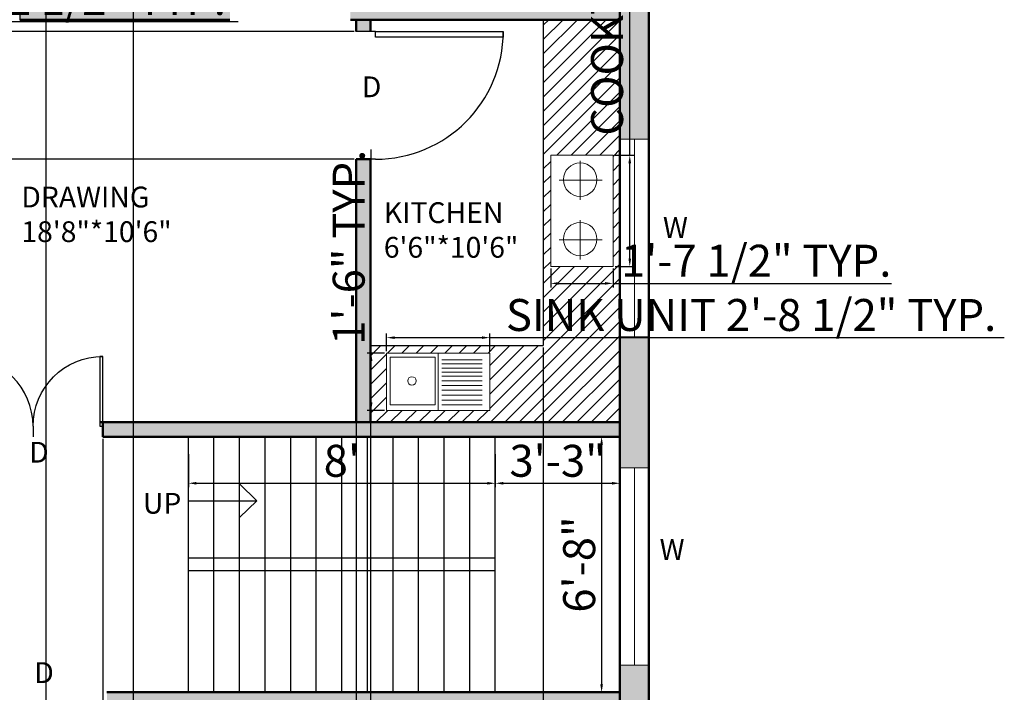
# Model space of a CAD drawing. Units: inches. Extents: x 1935 to 2445, y 1978 to 2806.
# Tile 3 of 4: x 2137 to 2445, y 2344 to 2554. Entities that reach past the tile are written whole.
import ezdxf

# ---------------------------------------------------------------- set-up
doc = ezdxf.new("R2010")
doc.units = ezdxf.units.IN
for name, color, linetype, lineweight in [('A-ANNO-DIMS', 2, 'Continuous', 18), ('A-ANNO-TEXT', 7, 'Continuous', 25), ('A-AREA-IDEN', 130, 'Continuous', 25), ('A-DOOR', 3, 'Continuous', 25), ('A-EQPM', 8, 'Continuous', 18), ('A-FLOR-CASE', 123, 'Continuous', 25), ('A-FLOR-CASE-PATT', 123, 'Continuous', 13), ('A-FLOR-FIXT', 9, 'Continuous', 18), ('A-FLOR-STRS', 7, 'Continuous', 25), ('A-GLAZ', 4, 'Continuous', 18), ('A-WALL-PATT', 225, 'Continuous', 13), ('WALL', 225, 'Continuous', 50)]:
    doc.layers.add(name, color=color, linetype=linetype, lineweight=lineweight)
doc.styles.get("Standard").update_dxf_attribs({"font": 'arial.ttf'})
doc.dimstyles.new('ISO-25', dxfattribs={"dimtxt": 10, "dimasz": 2.5, "dimexe": 1.25, "dimexo": 0.625, "dimtad": 1, "dimdec": 0, "dimlunit": 4, "dimtxsty": 'Standard', "dimcen": 2.5, "dimadec": 0, "dimazin": 0, "dimtfac": 1, "dimtdec": 0, "dimtmove": 0, "dimatfit": 3, "dimfxl": 1, "dimarcsym": 0})

# ---------------------------------------------------------------- blocks, each defined once
blk = doc.blocks.new('*U2')
for p, q in [((0, 0), (0, -6)), ((40, 0), (40, -6))]:
    blk.add_line(p, q)
blk.add_lwpolyline([(0, 0), (0, 40), (1.75, 40), (1.75, 0)], close=True)
blk.add_arc((0, 0), 40, 0, 90)
blk = doc.blocks.new('*D5')
at = {"layer": 'A-ANNO-DIMS', "color": 0, "lineweight": -2, "transparency": 16777216}
for p, q in [((2190.18, 2418.42), (2190.18, 2408.06)), ((2286.18, 2418.42), (2286.18, 2408.06)), ((2192.68, 2409.31), (2283.68, 2409.31))]:
    blk.add_line(p, q, dxfattribs=at)
at = {"layer": 'A-ANNO-DIMS', "color": 0, "lineweight": 100, "transparency": 16777216}
for points in [[(2192.68, 2409.72), (2192.68, 2408.89), (2190.18, 2409.31)], [(2283.68, 2409.72), (2283.68, 2408.89), (2286.18, 2409.31)]]:
    blk.add_solid(points, dxfattribs=at)
at = {"layer": 'Defpoints', "color": 0, "lineweight": 100, "transparency": 16777216}
for p in [(2190.18, 2419.04), (2286.18, 2419.04), (2286.18, 2409.31)]:
    blk.add_point(p, dxfattribs=at)
at = {"layer": 'A-ANNO-DIMS', "color": 0, "transparency": 16777216, "insert": (2238.18, 2415.04), "char_height": 10, "attachment_point": 5}
blk.add_mtext("8'", dxfattribs=at)
blk = doc.blocks.new('*D6')
at = {"layer": 'A-ANNO-DIMS', "color": 0, "lineweight": -2, "transparency": 16777216}
for p, q in [((2286.18, 2418.22), (2286.18, 2408.06)), ((2325.18, 2418.22), (2325.18, 2408.06)), ((2288.68, 2409.31), (2322.68, 2409.31))]:
    blk.add_line(p, q, dxfattribs=at)
at = {"layer": 'A-ANNO-DIMS', "color": 0, "lineweight": 100, "transparency": 16777216}
for points in [[(2288.68, 2409.72), (2288.68, 2408.89), (2286.18, 2409.31)], [(2322.68, 2409.72), (2322.68, 2408.89), (2325.18, 2409.31)]]:
    blk.add_solid(points, dxfattribs=at)
at = {"layer": 'Defpoints', "color": 0, "lineweight": 100, "transparency": 16777216}
for p in [(2286.18, 2418.85), (2325.18, 2418.85), (2325.18, 2409.31)]:
    blk.add_point(p, dxfattribs=at)
at = {"layer": 'A-ANNO-DIMS', "color": 0, "transparency": 16777216, "insert": (2305.68, 2415.04), "char_height": 10, "attachment_point": 5}
blk.add_mtext('3\'-3"', dxfattribs=at)
blk = doc.blocks.new('*D7')
at = {"layer": 'A-ANNO-DIMS', "color": 0, "lineweight": -2, "transparency": 16777216}
for p, q in [((2324.56, 2423.88), (2318.18, 2423.88)), ((2319.43, 2421.38), (2319.43, 2346.38)), ((2324.56, 2343.88), (2318.18, 2343.88))]:
    blk.add_line(p, q, dxfattribs=at)
at = {"layer": 'A-ANNO-DIMS', "color": 0, "lineweight": 100, "transparency": 16777216}
for points in [[(2319.01, 2421.38), (2319.85, 2421.38), (2319.43, 2423.88)], [(2319.01, 2346.38), (2319.85, 2346.38), (2319.43, 2343.88)]]:
    blk.add_solid(points, dxfattribs=at)
at = {"layer": 'Defpoints', "color": 0, "lineweight": 100, "transparency": 16777216}
for p in [(2325.18, 2423.88), (2319.43, 2343.88), (2325.18, 2343.88)]:
    blk.add_point(p, dxfattribs=at)
at = {"layer": 'A-ANNO-DIMS', "color": 0, "transparency": 16777216, "insert": (2313.7, 2383.88), "char_height": 10, "attachment_point": 5, "rotation": 90}
blk.add_mtext('6\'-8"', dxfattribs=at)
blk = doc.blocks.new('*D9')
at = {"layer": 'A-ANNO-DIMS', "color": 0, "lineweight": -2, "transparency": 16777216}
for p, q in [((2333.56, 2697.88), (1952.98, 2697.88)), ((1954.23, 2076.38), (1954.23, 2695.38)), ((2333.56, 2073.88), (1952.98, 2073.88))]:
    blk.add_line(p, q, dxfattribs=at)
at = {"layer": 'A-ANNO-DIMS', "color": 0, "lineweight": 100, "transparency": 16777216}
for points in [[(1953.82, 2695.38), (1954.65, 2695.38), (1954.23, 2697.88)], [(1953.82, 2076.38), (1954.65, 2076.38), (1954.23, 2073.88)]]:
    blk.add_solid(points, dxfattribs=at)
at = {"layer": 'Defpoints', "color": 0, "lineweight": 100, "transparency": 16777216}
for p in [(1954.23, 2697.88), (2334.18, 2697.88), (2334.18, 2073.88)]:
    blk.add_point(p, dxfattribs=at)
at = {"layer": 'A-ANNO-DIMS', "color": 0, "transparency": 16777216, "insert": (1948.5, 2385.88), "char_height": 10, "attachment_point": 5, "rotation": 90}
blk.add_mtext("52'", dxfattribs=at)
blk = doc.blocks.new('WINDOW-STD')
blk.add_line((0, 4.5), (61.82, 4.5))
blk.add_lwpolyline([(0, 9), (61.82, 9), (61.82, 0), (0, 0)], close=True)
blk = doc.blocks.new('SINK-WITH-DRAINBOARD')
for p, q in [((16.15, 17.9), (16.15, 0)), ((17.28, 15.79), (29.84, 15.79)), ((17.28, 14.55), (29.84, 14.55)), ((17.28, 13.18), (29.84, 13.18)), ((17.28, 11.91), (29.84, 11.91)), ((17.28, 10.66), (29.84, 10.66)), ((17.28, 9.26), (29.84, 9.26)), ((17.28, 7.74), (29.84, 7.74)), ((17.28, 6.29), (29.84, 6.29)), ((17.28, 4.78), (29.84, 4.78)), ((17.28, 3.21), (29.84, 3.21)), ((17.28, 1.68), (29.84, 1.68))]:
    blk.add_line(p, q)
for points in [[(0, 17.9), (32.3, 17.9), (32.3, 0), (0, 0)], [(1.08, 1.69), (15.15, 1.69), (15.15, 16.69), (1.08, 16.69)]]:
    blk.add_lwpolyline(points, close=True)
blk.add_circle((7.93, 9.19), 1.34)
blk = doc.blocks.new('COOKTOP-2-BURNER')
for p, q in [((9.23, 27.22), (9.23, 33.16)), ((9.23, 33.16), (9.23, 20.87)), ((9.23, 27.02), (2.64, 27.02)), ((2.64, 27.02), (16.07, 27.02)), ((9.23, 20.87), (9.23, 27.02)), ((9.23, 8.61), (9.23, 14.56)), ((9.23, 14.56), (9.23, 2.26)), ((9.23, 8.41), (2.64, 8.41)), ((2.64, 8.41), (16.07, 8.41)), ((9.23, 2.26), (9.23, 8.41))]:
    blk.add_line(p, q)
blk.add_lwpolyline([(0, 34.88), (19.51, 34.88), (19.51, 0), (0, 0)], close=True)
for centre in [(9.23, 27.22), (9.23, 8.61)]:
    blk.add_circle(centre, 5.23)
blk = doc.blocks.new('*D26')
at = {"layer": 'A-ANNO-DIMS', "color": 0, "lineweight": -2, "transparency": 16777216}
for p, q in [((2022.21, 2552.24), (2022.21, 2555.04)), ((2024.71, 2553.79), (2034.22, 2553.79)), ((2036.72, 2552.24), (2036.72, 2555.04)), ((2036.72, 2553.79), (2205.72, 2553.79))]:
    blk.add_line(p, q, dxfattribs=at)
at = {"layer": 'A-ANNO-DIMS', "color": 0, "lineweight": 100, "transparency": 16777216}
for points in [[(2024.71, 2554.21), (2024.71, 2553.37), (2022.21, 2553.79)], [(2034.22, 2554.21), (2034.22, 2553.37), (2036.72, 2553.79)]]:
    blk.add_solid(points, dxfattribs=at)
at = {"layer": 'Defpoints', "color": 0, "lineweight": 100, "transparency": 16777216}
for p in [(2036.72, 2553.79), (2022.21, 2551.61), (2036.72, 2551.61)]:
    blk.add_point(p, dxfattribs=at)
at = {"layer": 'A-ANNO-DIMS', "color": 0, "transparency": 16777216, "insert": (2122.47, 2559.59), "char_height": 10, "attachment_point": 5}
blk.add_mtext('END TABLE 1\'-2 1/2" TYP.', dxfattribs=at)
blk = doc.blocks.new('*D30')
at = {"layer": 'A-ANNO-DIMS', "color": 0, "lineweight": -2, "transparency": 16777216}
for p, q in [((2252.19, 2450.66), (2252.19, 2456.13)), ((2254.69, 2454.88), (2281.98, 2454.88)), ((2284.48, 2450.66), (2284.48, 2456.13)), ((2284.48, 2454.88), (2445.4, 2454.88))]:
    blk.add_line(p, q, dxfattribs=at)
at = {"layer": 'A-ANNO-DIMS', "color": 0, "lineweight": 100, "transparency": 16777216}
for points in [[(2254.69, 2455.29), (2254.69, 2454.46), (2252.19, 2454.88)], [(2281.98, 2455.29), (2281.98, 2454.46), (2284.48, 2454.88)]]:
    blk.add_solid(points, dxfattribs=at)
at = {"layer": 'Defpoints', "color": 0, "lineweight": 100, "transparency": 16777216}
for p in [(2284.48, 2454.88), (2252.19, 2450.03), (2284.48, 2450.03)]:
    blk.add_point(p, dxfattribs=at)
at = {"layer": 'A-ANNO-DIMS', "color": 0, "transparency": 16777216, "insert": (2366.19, 2460.67), "char_height": 10, "attachment_point": 5}
blk.add_mtext('SINK UNIT 2\'-8 1/2" TYP.', dxfattribs=at)
blk = doc.blocks.new('*D31')
at = {"layer": 'A-ANNO-DIMS', "color": 0, "lineweight": -2, "transparency": 16777216}
for p, q in [((2247.34, 2450.03), (2247.34, 2513.79)), ((2251.56, 2450.03), (2246.09, 2450.03)), ((2247.34, 2434.63), (2247.34, 2447.53)), ((2251.56, 2432.13), (2246.09, 2432.13))]:
    blk.add_line(p, q, dxfattribs=at)
at = {"layer": 'A-ANNO-DIMS', "color": 0, "lineweight": 100, "transparency": 16777216}
for points in [[(2246.92, 2447.53), (2247.76, 2447.53), (2247.34, 2450.03)], [(2246.92, 2434.63), (2247.76, 2434.63), (2247.34, 2432.13)]]:
    blk.add_solid(points, dxfattribs=at)
at = {"layer": 'Defpoints', "color": 0, "lineweight": 100, "transparency": 16777216}
for p in [(2247.34, 2450.03), (2252.19, 2450.03), (2252.19, 2432.13)]:
    blk.add_point(p, dxfattribs=at)
at = {"layer": 'A-ANNO-DIMS', "color": 0, "transparency": 16777216, "insert": (2241.61, 2483.16), "char_height": 10, "attachment_point": 5, "rotation": 90}
blk.add_mtext('1\'-6" TYP.', dxfattribs=at)
blk = doc.blocks.new('*D32')
at = {"layer": 'A-ANNO-DIMS', "color": 0, "lineweight": -2, "transparency": 16777216}
for p, q in [((2328.24, 2511.98), (2328.24, 2658.07)), ((2323.63, 2511.98), (2329.49, 2511.98)), ((2328.24, 2479.6), (2328.24, 2509.48)), ((2323.63, 2477.1), (2329.49, 2477.1))]:
    blk.add_line(p, q, dxfattribs=at)
at = {"layer": 'A-ANNO-DIMS', "color": 0, "lineweight": 100, "transparency": 16777216}
for points in [[(2327.82, 2509.48), (2328.66, 2509.48), (2328.24, 2511.98)], [(2327.82, 2479.6), (2328.66, 2479.6), (2328.24, 2477.1)]]:
    blk.add_solid(points, dxfattribs=at)
at = {"layer": 'Defpoints', "color": 0, "lineweight": 100, "transparency": 16777216}
for p in [(2323.01, 2511.98), (2328.24, 2511.98), (2323.01, 2477.1)]:
    blk.add_point(p, dxfattribs=at)
at = {"layer": 'A-ANNO-DIMS', "color": 0, "transparency": 16777216, "insert": (2322.44, 2586.27), "char_height": 10, "attachment_point": 5, "rotation": 90}
blk.add_mtext('COOKTOP 2\'-11" TYP.', dxfattribs=at)
blk = doc.blocks.new('*D33')
at = {"layer": 'A-ANNO-DIMS', "color": 0, "lineweight": -2, "transparency": 16777216}
for p, q in [((2303.5, 2476.47), (2303.5, 2470.61)), ((2323.01, 2476.47), (2323.01, 2470.61)), ((2306, 2471.86), (2320.51, 2471.86)), ((2323.01, 2471.86), (2410.07, 2471.86))]:
    blk.add_line(p, q, dxfattribs=at)
at = {"layer": 'A-ANNO-DIMS', "color": 0, "lineweight": 100, "transparency": 16777216}
for points in [[(2306, 2472.28), (2306, 2471.45), (2303.5, 2471.86)], [(2320.51, 2472.28), (2320.51, 2471.45), (2323.01, 2471.86)]]:
    blk.add_solid(points, dxfattribs=at)
at = {"layer": 'Defpoints', "color": 0, "lineweight": 100, "transparency": 16777216}
for p in [(2303.5, 2477.1), (2323.01, 2477.1), (2323.01, 2471.86)]:
    blk.add_point(p, dxfattribs=at)
at = {"layer": 'A-ANNO-DIMS', "color": 0, "transparency": 16777216, "insert": (2367.79, 2477.66), "char_height": 10, "attachment_point": 5}
blk.add_mtext('1\'-7 1/2" TYP.', dxfattribs=at)
blk = doc.blocks.new('*D40')
at = {"layer": 'A-ANNO-DIMS', "color": 0, "lineweight": -2, "transparency": 16777216}
for p, q in [((2119.73, 2423.26), (2119.73, 1986.08)), ((2163.45, 2423.26), (2163.45, 1986.08)), ((2122.23, 1987.33), (2160.95, 1987.33)), ((2163.45, 1987.33), (2217.08, 1987.33))]:
    blk.add_line(p, q, dxfattribs=at)
at = {"layer": 'A-ANNO-DIMS', "color": 0, "lineweight": 100, "transparency": 16777216}
for points in [[(2122.23, 1987.74), (2122.23, 1986.91), (2119.73, 1987.33)], [(2160.95, 1987.74), (2160.95, 1986.91), (2163.45, 1987.33)]]:
    blk.add_solid(points, dxfattribs=at)
at = {"layer": 'Defpoints', "color": 0, "lineweight": 100, "transparency": 16777216}
for p in [(2119.73, 2423.88), (2163.45, 2423.88), (2163.45, 1987.33)]:
    blk.add_point(p, dxfattribs=at)
at = {"layer": 'A-ANNO-DIMS', "color": 0, "transparency": 16777216, "insert": (2191.52, 1993.13), "char_height": 10, "attachment_point": 5}
blk.add_mtext('3\'-7 1/2"', dxfattribs=at)
blk = doc.blocks.new('*D42')
at = {"layer": 'A-ANNO-DIMS', "color": 0, "lineweight": -2, "transparency": 16777216}
for p, q in [((2145.55, 2591.86), (2145.55, 1986.08)), ((2172.86, 2592.26), (2172.86, 1986.08)), ((2148.05, 1987.33), (2170.36, 1987.33)), ((2172.86, 1987.33), (2226.66, 1987.33))]:
    blk.add_line(p, q, dxfattribs=at)
at = {"layer": 'A-ANNO-DIMS', "color": 0, "lineweight": 100, "transparency": 16777216}
for points in [[(2148.05, 1987.74), (2148.05, 1986.91), (2145.55, 1987.33)], [(2170.36, 1987.74), (2170.36, 1986.91), (2172.86, 1987.33)]]:
    blk.add_solid(points, dxfattribs=at)
at = {"layer": 'Defpoints', "color": 0, "lineweight": 100, "transparency": 16777216}
for p in [(2145.55, 2592.49), (2172.86, 2592.88), (2172.86, 1987.33)]:
    blk.add_point(p, dxfattribs=at)
at = {"layer": 'A-ANNO-DIMS', "color": 0, "transparency": 16777216, "insert": (2201.01, 1993.13), "char_height": 10, "attachment_point": 5}
blk.add_mtext('2\'-3 1/2"', dxfattribs=at)
blk = doc.blocks.new('*D43')
at = {"layer": 'A-ANNO-DIMS', "color": 0, "lineweight": -2, "transparency": 16777216}
for p, q in [((2242.06, 2550.71), (1964.13, 2550.71)), ((1965.38, 2513.21), (1965.38, 2548.21)), ((2242.06, 2510.71), (1964.13, 2510.71))]:
    blk.add_line(p, q, dxfattribs=at)
at = {"layer": 'A-ANNO-DIMS', "color": 0, "lineweight": 100, "transparency": 16777216}
for points in [[(1964.96, 2548.21), (1965.8, 2548.21), (1965.38, 2550.71)], [(1964.96, 2513.21), (1965.8, 2513.21), (1965.38, 2510.71)]]:
    blk.add_solid(points, dxfattribs=at)
at = {"layer": 'Defpoints', "color": 0, "lineweight": 100, "transparency": 16777216}
for p in [(1965.38, 2550.71), (2242.68, 2550.71), (2242.68, 2510.71)]:
    blk.add_point(p, dxfattribs=at)
at = {"layer": 'A-ANNO-DIMS', "color": 0, "transparency": 16777216, "insert": (1959.65, 2530.71), "char_height": 10, "attachment_point": 5, "rotation": 90}
blk.add_mtext('3\'-4"', dxfattribs=at)
blk = doc.blocks.new('*D44')
at = {"layer": 'A-ANNO-DIMS', "color": 0, "lineweight": -2, "transparency": 16777216}
for p, q in [((2301.18, 2451.76), (2301.18, 1986.08)), ((2325.18, 2454.54), (2325.18, 1986.08)), ((2303.68, 1987.33), (2322.68, 1987.33)), ((2325.18, 1987.33), (2355.69, 1987.33))]:
    blk.add_line(p, q, dxfattribs=at)
at = {"layer": 'A-ANNO-DIMS', "color": 0, "lineweight": 100, "transparency": 16777216}
for points in [[(2303.68, 1987.74), (2303.68, 1986.91), (2301.18, 1987.33)], [(2322.68, 1987.74), (2322.68, 1986.91), (2325.18, 1987.33)]]:
    blk.add_solid(points, dxfattribs=at)
at = {"layer": 'Defpoints', "color": 0, "lineweight": 100, "transparency": 16777216}
for p in [(2325.18, 2455.16), (2301.18, 2452.38), (2325.18, 1987.33)]:
    blk.add_point(p, dxfattribs=at)
at = {"layer": 'A-ANNO-DIMS', "color": 0, "transparency": 16777216, "insert": (2341.69, 1993.06), "char_height": 10, "attachment_point": 5}
blk.add_mtext('2\'-0"', dxfattribs=at)
blk = doc.blocks.new('*D45')
at = {"layer": 'A-ANNO-DIMS', "color": 0, "lineweight": -2, "transparency": 16777216}
for p, q in [((2242.68, 2510.08), (2242.68, 1986.08)), ((2247.18, 2510.08), (2247.18, 1986.08)), ((2240.18, 1987.33), (2237.68, 1987.33)), ((2242.68, 1987.33), (2247.18, 1987.33)), ((2249.68, 1987.33), (2303.32, 1987.33))]:
    blk.add_line(p, q, dxfattribs=at)
at = {"layer": 'A-ANNO-DIMS', "color": 0, "lineweight": 100, "transparency": 16777216}
for points in [[(2240.18, 1987.74), (2240.18, 1986.91), (2242.68, 1987.33)], [(2249.68, 1987.74), (2249.68, 1986.91), (2247.18, 1987.33)]]:
    blk.add_solid(points, dxfattribs=at)
at = {"layer": 'Defpoints', "color": 0, "lineweight": 100, "transparency": 16777216}
for p in [(2242.68, 2510.71), (2247.18, 2510.71), (2247.18, 1987.33)]:
    blk.add_point(p, dxfattribs=at)
at = {"layer": 'A-ANNO-DIMS', "color": 0, "transparency": 16777216, "insert": (2277.75, 1993.12), "char_height": 10, "attachment_point": 5}
blk.add_mtext('0\'-4 1/2"', dxfattribs=at)

msp = doc.modelspace()

# ---------------------------------------------------------------- hatches: boundary and pattern name
at = {"layer": 'A-FLOR-CASE-PATT'}
h = msp.add_hatch(dxfattribs=at)
h.set_pattern_fill('ANSI31', color=256)
h.paths.add_polyline_path([(2325.18, 2339.38), (2286.18, 2339.38), (2247.18, 2339.38), (2247.18, 2315.38), (2301.18, 2315.38), (2301.18, 2213.38), (2325.18, 2213.38)])
h.paths.add_polyline_path([(2284.48, 2318.31), (2252.19, 2318.31), (2252.19, 2336.21), (2284.48, 2336.21)], flags=16)
h.paths.add_polyline_path([(2303.5, 2299.32), (2323.01, 2299.32), (2323.01, 2264.44), (2303.5, 2264.44)], flags=16)
h.paths.add_polyline_path([(2317.96, 2291.66, -1), (2307.51, 2291.66, -1)], flags=0)
h.paths.add_polyline_path([(2267.33, 2320), (2253.26, 2320), (2253.26, 2335.01), (2267.33, 2335.01)], flags=0)
h.paths.add_polyline_path([(2258.78, 2327.5, -1), (2261.46, 2327.5, -1)], flags=0)
h.paths.add_polyline_path([(2317.96, 2273.05, -1), (2307.51, 2273.05, -1)], flags=0)
h.paths.add_polyline_path([(2325.18, 2554.38), (2301.18, 2554.38), (2301.18, 2452.38), (2247.18, 2452.38), (2247.18, 2428.38), (2325.18, 2428.38)])
h.paths.add_polyline_path([(2323.01, 2511.98), (2323.01, 2477.1), (2303.5, 2477.1), (2303.5, 2511.98)], flags=16)
h.paths.add_polyline_path([(2317.96, 2504.31, -1), (2307.51, 2504.31, -1)], flags=0)
h.paths.add_polyline_path([(2317.96, 2485.7, -1), (2307.51, 2485.7, -1)], flags=0)
h.paths.add_polyline_path([(2284.48, 2450.03), (2284.48, 2432.13), (2252.19, 2432.13), (2252.19, 2450.03)], flags=16)
h.paths.add_polyline_path([(2267.33, 2448.82), (2267.33, 2433.82), (2253.26, 2433.82), (2253.26, 2448.82)], flags=0)
h.paths.add_polyline_path([(2261.46, 2441.32, -1), (2258.78, 2441.32, -1)], flags=0)
at = {"layer": 'A-WALL-PATT'}
h = msp.add_hatch(color=256, dxfattribs=at)
h.dxf.hatch_style = 1
h.paths.add_polyline_path([(2047.95, 2697.88), (2010.18, 2697.88), (2010.18, 2654.96), (2019.18, 2654.96), (2019.18, 2688.88), (2047.95, 2688.88)], flags=16)
h.paths.add_polyline_path([(2156.17, 2697.88), (2109.77, 2697.88), (2109.77, 2688.88), (2139.18, 2688.88), (2156.17, 2688.88)], flags=17)
h.paths.add_polyline_path([(2231.53, 2697.88), (2186.46, 2697.88), (2186.46, 2688.88), (2231.53, 2688.88)], flags=17)
h.paths.add_polyline_path([(2334.18, 2697.88), (2293.35, 2697.88), (2293.35, 2688.88), (2325.18, 2688.88), (2325.18, 2651.52), (2334.18, 2651.52)], flags=17)
h.paths.add_polyline_path([(2247.18, 2554.38), (2242.68, 2554.38), (2242.68, 2550.71), (2247.18, 2550.71)], flags=17)
h.paths.add_polyline_path([(2145.55, 2592.49), (2145.55, 2592.88), (2143.68, 2592.88), (2143.68, 2588.39), (2145.55, 2588.39)], flags=17)
h.paths.add_polyline_path([(2197.68, 2592.88), (2172.86, 2592.88, -0.003651), (2172.86, 2592.49), (2172.86, 2588.39), (2197.68, 2588.39)], flags=17)
h.paths.add_polyline_path([(2203.16, 2558.88), (2137.4, 2558.88), (2137.4, 2554.38), (2143.68, 2554.38), (2203.16, 2554.38)], flags=17)
h.paths.add_polyline_path([(2097.4, 2558.88), (2019.18, 2558.88), (2019.18, 2554.38), (2097.4, 2554.38)], flags=17)
h.paths.add_polyline_path([(2143.68, 2688.88), (2139.18, 2688.88), (2139.18, 2558.88), (2143.68, 2558.88)], flags=17)
h.paths.add_polyline_path([(2202.18, 2688.88), (2197.68, 2688.88), (2197.68, 2592.88), (2197.68, 2588.39), (2197.68, 2558.88), (2202.18, 2558.88), (2202.18, 2588.38)], flags=17)
h.paths.add_polyline_path([(2241.74, 2229.79), (2251.55, 2229.79), (2251.55, 2243.19), (2241.74, 2243.19)], flags=25)
h.paths.add_polyline_path([(2215.53, 2200.14), (2225.34, 2200.14), (2225.34, 2213.54), (2215.53, 2213.54)], flags=25)
h.paths.add_polyline_path([(2152.61, 2173.98), (2162.42, 2173.98), (2162.42, 2187.38), (2152.61, 2187.38)], flags=25)
h.paths.add_polyline_path([(2109.99, 2200.78), (2119.8, 2200.78), (2119.8, 2214.18), (2109.99, 2214.18)], flags=25)
h.paths.add_polyline_path([(2139.65, 2343.23), (2149.46, 2343.23), (2149.46, 2356.63), (2139.65, 2356.63)], flags=25)
h.paths.add_polyline_path([(2138.05, 2412.22), (2147.87, 2412.22), (2147.87, 2425.62), (2138.05, 2425.62)], flags=25)
h.paths.add_polyline_path([(2242.1, 2526.57), (2251.91, 2526.57), (2251.91, 2539.97), (2242.1, 2539.97)], flags=25)
h.paths.add_polyline_path([(2212.92, 2555.35), (2222.74, 2555.35), (2222.74, 2568.75), (2212.92, 2568.75)], flags=25)
h.paths.add_polyline_path([(2111.94, 2553.1), (2121.75, 2553.1), (2121.75, 2566.5), (2111.94, 2566.5)], flags=25)
h.paths.add_polyline_path([(2032.85, 2161.17), (2083.36, 2161.17), (2083.36, 2185.43), (2032.85, 2185.43)], flags=25)
h.paths.add_polyline_path([(2145.49, 2119.25), (2193.41, 2119.25), (2193.41, 2143.52), (2145.49, 2143.52)], flags=25)
h.paths.add_polyline_path([(2250.93, 2163.1), (2301.44, 2163.1), (2301.44, 2187.36), (2250.93, 2187.36)], flags=25)
h.paths.add_polyline_path([(2247.75, 2274.43), (2290.88, 2274.43), (2290.88, 2298.69), (2247.75, 2298.69)], flags=25)
h.paths.add_polyline_path([(2131.26, 2265.2), (2178.71, 2265.2), (2178.71, 2289.46), (2131.26, 2289.46)], flags=25)
h.paths.add_polyline_path([(2092.71, 2400.61), (2092.71, 2376.16), (2106.11, 2376.16), (2106.11, 2400.61)], flags=25)
h.paths.add_polyline_path([(2173.61, 2396.23), (2189.48, 2396.23), (2189.48, 2409.63), (2173.61, 2409.63)], flags=25)
h.paths.add_polyline_path([(2028.85, 2376.01), (2076.42, 2376.01), (2076.42, 2400.28), (2028.85, 2400.28)], flags=25)
h.paths.add_polyline_path([(2135.3, 2481.1), (2182.75, 2481.1), (2182.75, 2505.37), (2135.3, 2505.37)], flags=25)
h.paths.add_polyline_path([(2249.01, 2476.21), (2292.13, 2476.21), (2292.13, 2500.47), (2249.01, 2500.47)], flags=25)
h.paths.add_polyline_path([(2251.9, 2596.84), (2302.42, 2596.84), (2302.42, 2621.11), (2251.9, 2621.11)], flags=25)
h.paths.add_polyline_path([(2030.66, 2589.83), (2081.18, 2589.83), (2081.18, 2614.09), (2030.66, 2614.09)], flags=25)
h.paths.add_polyline_path([(2019.18, 2593.14), (2010.18, 2593.14), (2010.18, 2520.31), (2019.18, 2520.31)])
h.paths.add_polyline_path([(2010.18, 2164.99), (2019.18, 2164.99), (2019.18, 2238.56), (2010.18, 2238.56)])
h.paths.add_polyline_path([(2048.33, 2073.88), (2048.33, 2082.88), (2019.18, 2082.88), (2019.18, 2103.18), (2010.18, 2103.18), (2010.18, 2073.88)])
h.paths.add_polyline_path([(2156.55, 2073.88), (2156.55, 2082.88), (2110.15, 2082.88), (2110.15, 2073.88)])
h.paths.add_polyline_path([(2231.91, 2073.88), (2231.91, 2082.88), (2186.84, 2082.88), (2186.84, 2073.88)])
h.paths.add_polyline_path([(2047.95, 2688.88), (2047.95, 2697.88), (2010.18, 2697.88), (2010.18, 2654.96), (2019.18, 2654.96), (2019.18, 2688.88)])
h.paths.add_polyline_path([(2109.77, 2697.88), (2109.77, 2688.88), (2156.17, 2688.88), (2156.17, 2697.88)])
h = msp.add_hatch(color=256, dxfattribs=at)
h.dxf.hatch_style = 1
h.paths.add_polyline_path([(2196.68, 2183.38), (2171.78, 2183.38), (2171.78, 2179.29, -0.003687), (2171.78, 2178.88), (2196.68, 2178.88)], flags=17)
h.paths.add_polyline_path([(2144.47, 2183.38), (2142.68, 2183.38), (2142.68, 2178.88), (2144.47, 2178.88), (2144.47, 2179.29)], flags=17)
h.paths.add_polyline_path([(2096.62, 2213.38), (2019.18, 2213.38), (2019.18, 2208.88), (2096.62, 2208.88)], flags=17)
h.paths.add_polyline_path([(2142.68, 2208.88), (2142.68, 2213.38), (2136.62, 2213.38), (2136.62, 2208.88), (2138.18, 2208.88), (2138.18, 2183.38), (2138.18, 2082.88), (2142.68, 2082.88), (2142.68, 2178.88), (2142.68, 2183.38)], flags=17)
h.paths.add_polyline_path([(2201.18, 2208.88), (2202.06, 2208.88), (2202.06, 2213.38), (2196.68, 2213.38), (2196.68, 2204.97), (2196.68, 2082.88), (2201.18, 2082.88)], flags=17)
h.paths.add_polyline_path([(2247.18, 2217.21), (2242.68, 2217.21), (2242.68, 2213.38), (2247.18, 2213.38)], flags=17)
h.paths.add_polyline_path([(2325.18, 2213.38), (2242.68, 2213.38), (2242.68, 2208.88), (2325.18, 2208.88)], flags=17)
h.paths.add_polyline_path([(2247.18, 2339.38), (2242.68, 2339.38), (2242.68, 2257.21), (2247.18, 2257.21)], flags=17)
h.paths.add_polyline_path([(2325.18, 2343.88), (2286.18, 2343.88), (2186.18, 2343.88), (2164.69, 2343.88), (2164.69, 2340.61), (2164.69, 2339.38), (2213.9, 2339.38), (2286.18, 2339.38), (2325.18, 2339.38)], flags=17)
h.paths.add_polyline_path([(2109.68, 2343.88), (2105.18, 2343.88), (2019.18, 2343.88), (2019.18, 2339.38), (2109.68, 2339.38)], flags=17)
h.paths.add_polyline_path([(2120.97, 2340.61), (2120.97, 2343.88), (2109.68, 2343.88), (2109.68, 2339.38), (2120.97, 2339.38)], flags=17)
h.paths.add_polyline_path([(2109.68, 2356.84), (2105.18, 2356.84), (2105.18, 2343.88), (2109.68, 2343.88)], flags=17)
h.paths.add_polyline_path([(2230.51, 2409.48), (2245.95, 2409.48), (2245.95, 2430.09), (2230.51, 2430.09)], flags=25)
h.paths.add_polyline_path([(2289.31, 2409.69), (2322.13, 2409.69), (2322.13, 2430.3), (2289.31, 2430.3)], flags=25)
h.paths.add_polyline_path([(2241.74, 2229.79), (2251.55, 2229.79), (2251.55, 2243.19), (2241.74, 2243.19)], flags=25)
h.paths.add_polyline_path([(2215.53, 2200.14), (2225.34, 2200.14), (2225.34, 2213.54), (2215.53, 2213.54)], flags=25)
h.paths.add_polyline_path([(2152.61, 2173.98), (2162.42, 2173.98), (2162.42, 2187.38), (2152.61, 2187.38)], flags=25)
h.paths.add_polyline_path([(2109.99, 2200.78), (2119.8, 2200.78), (2119.8, 2214.18), (2109.99, 2214.18)], flags=25)
h.paths.add_polyline_path([(2139.65, 2343.23), (2149.46, 2343.23), (2149.46, 2356.63), (2139.65, 2356.63)], flags=25)
h.paths.add_polyline_path([(2138.05, 2412.22), (2147.87, 2412.22), (2147.87, 2425.62), (2138.05, 2425.62)], flags=25)
h.paths.add_polyline_path([(2242.1, 2526.57), (2251.91, 2526.57), (2251.91, 2539.97), (2242.1, 2539.97)], flags=25)
h.paths.add_polyline_path([(2212.92, 2555.35), (2222.74, 2555.35), (2222.74, 2568.75), (2212.92, 2568.75)], flags=25)
h.paths.add_polyline_path([(2151.96, 2587.49), (2161.77, 2587.49), (2161.77, 2600.89), (2151.96, 2600.89)], flags=25)
h.paths.add_polyline_path([(2111.94, 2553.1), (2121.75, 2553.1), (2121.75, 2566.5), (2111.94, 2566.5)], flags=25)
h.paths.add_polyline_path([(2032.85, 2161.17), (2083.36, 2161.17), (2083.36, 2185.43), (2032.85, 2185.43)], flags=25)
h.paths.add_polyline_path([(2145.49, 2119.25), (2193.41, 2119.25), (2193.41, 2143.52), (2145.49, 2143.52)], flags=25)
h.paths.add_polyline_path([(2250.93, 2163.1), (2301.44, 2163.1), (2301.44, 2187.36), (2250.93, 2187.36)], flags=25)
h.paths.add_polyline_path([(2247.75, 2274.43), (2290.88, 2274.43), (2290.88, 2298.69), (2247.75, 2298.69)], flags=25)
h.paths.add_polyline_path([(2131.26, 2265.2), (2178.71, 2265.2), (2178.71, 2289.46), (2131.26, 2289.46)], flags=25)
h.paths.add_polyline_path([(2173.61, 2396.23), (2189.48, 2396.23), (2189.48, 2409.63), (2173.61, 2409.63)], flags=25)
h.paths.add_polyline_path([(2135.3, 2481.1), (2182.75, 2481.1), (2182.75, 2505.37), (2135.3, 2505.37)], flags=25)
h.paths.add_polyline_path([(2249.01, 2476.21), (2292.13, 2476.21), (2292.13, 2500.47), (2249.01, 2500.47)], flags=25)
h.paths.add_polyline_path([(2251.9, 2596.84), (2302.42, 2596.84), (2302.42, 2621.11), (2251.9, 2621.11)], flags=25)
h.paths.add_polyline_path([(2148.05, 2628.52), (2195.98, 2628.52), (2195.98, 2652.78), (2148.05, 2652.78)], flags=25)
h.paths.add_polyline_path([(2030.66, 2589.83), (2081.18, 2589.83), (2081.18, 2614.09), (2030.66, 2614.09)], flags=25)
h.paths.add_polyline_path([(2325.18, 2414.18), (2334.18, 2414.18), (2334.18, 2455.16), (2325.18, 2455.16)])
h.paths.add_polyline_path([(2325.18, 2305.65), (2334.18, 2305.65), (2334.18, 2352.36), (2325.18, 2352.36)])
h.paths.add_polyline_path([(2325.18, 2163.2), (2334.18, 2163.2), (2334.18, 2243.83), (2325.18, 2243.83)])
h.paths.add_polyline_path([(2293.73, 2082.88), (2293.73, 2073.88), (2334.18, 2073.88), (2334.18, 2101.39), (2325.18, 2101.39), (2325.18, 2082.88)])
h.paths.add_polyline_path([(2334.18, 2589.71), (2325.18, 2589.71), (2325.18, 2516.98), (2334.18, 2516.98)])
h.paths.add_polyline_path([(2293.35, 2697.88), (2293.35, 2688.88), (2325.18, 2688.88), (2325.18, 2651.52), (2334.18, 2651.52), (2334.18, 2697.88)])
h.paths.add_polyline_path([(2109.77, 2697.88), (2109.77, 2688.88), (2231.53, 2688.88), (2231.53, 2697.88)])
h.paths.add_polyline_path([(2010.18, 2654.96), (2019.18, 2654.96), (2019.18, 2688.88), (2047.95, 2688.88), (2047.95, 2697.88), (2010.18, 2697.88)])
h.paths.add_polyline_path([(2010.18, 2520.31), (2019.18, 2520.31), (2019.18, 2593.14), (2010.18, 2593.14)])
h = msp.add_hatch(color=256, dxfattribs=at)
h.dxf.hatch_style = 1
h.paths.add_polyline_path([(2334.18, 2589.71), (2325.18, 2589.71), (2325.18, 2516.98), (2334.18, 2516.98)])
h.paths.add_polyline_path([(2325.18, 2558.88), (2240.84, 2558.88), (2240.84, 2554.38), (2325.18, 2554.38)])
h.paths.add_polyline_path([(2119.73, 2427.16), (2119.73, 2428.38), (2019.18, 2428.38), (2019.18, 2423.88), (2119.73, 2423.88)])
h.paths.add_polyline_path([(2230.51, 2409.48), (2245.95, 2409.48), (2245.95, 2430.09), (2230.51, 2430.09)], flags=9)
h.paths.add_polyline_path([(2289.31, 2409.69), (2322.13, 2409.69), (2322.13, 2430.3), (2289.31, 2430.3)], flags=9)
h.paths.add_polyline_path([(2241.74, 2229.79), (2251.55, 2229.79), (2251.55, 2243.19), (2241.74, 2243.19)], flags=9)
h.paths.add_polyline_path([(2215.53, 2200.14), (2225.34, 2200.14), (2225.34, 2213.54), (2215.53, 2213.54)], flags=9)
h.paths.add_polyline_path([(2152.61, 2173.98), (2162.42, 2173.98), (2162.42, 2187.38), (2152.61, 2187.38)], flags=9)
h.paths.add_polyline_path([(2109.99, 2200.78), (2119.8, 2200.78), (2119.8, 2214.18), (2109.99, 2214.18)], flags=9)
h.paths.add_polyline_path([(2139.65, 2343.23), (2149.46, 2343.23), (2149.46, 2356.63), (2139.65, 2356.63)], flags=9)
h.paths.add_polyline_path([(2138.05, 2412.22), (2147.87, 2412.22), (2147.87, 2425.62), (2138.05, 2425.62)], flags=9)
h.paths.add_polyline_path([(2242.1, 2526.57), (2251.91, 2526.57), (2251.91, 2539.97), (2242.1, 2539.97)], flags=9)
h.paths.add_polyline_path([(2212.92, 2555.35), (2222.74, 2555.35), (2222.74, 2568.75), (2212.92, 2568.75)], flags=9)
h.paths.add_polyline_path([(2151.96, 2587.49), (2161.77, 2587.49), (2161.77, 2600.89), (2151.96, 2600.89)], flags=9)
h.paths.add_polyline_path([(2111.94, 2553.1), (2121.75, 2553.1), (2121.75, 2566.5), (2111.94, 2566.5)], flags=9)
h.paths.add_polyline_path([(2032.85, 2161.17), (2083.36, 2161.17), (2083.36, 2185.43), (2032.85, 2185.43)], flags=9)
h.paths.add_polyline_path([(2145.49, 2119.25), (2193.41, 2119.25), (2193.41, 2143.52), (2145.49, 2143.52)], flags=9)
h.paths.add_polyline_path([(2250.93, 2163.1), (2301.44, 2163.1), (2301.44, 2187.36), (2250.93, 2187.36)], flags=9)
h.paths.add_polyline_path([(2247.75, 2274.43), (2290.88, 2274.43), (2290.88, 2298.69), (2247.75, 2298.69)], flags=9)
h.paths.add_polyline_path([(2131.26, 2265.2), (2178.71, 2265.2), (2178.71, 2289.46), (2131.26, 2289.46)], flags=9)
h.paths.add_polyline_path([(2173.61, 2396.23), (2189.48, 2396.23), (2189.48, 2409.63), (2173.61, 2409.63)], flags=9)
h.paths.add_polyline_path([(2135.3, 2481.1), (2182.75, 2481.1), (2182.75, 2505.37), (2135.3, 2505.37)], flags=9)
h.paths.add_polyline_path([(2249.01, 2476.21), (2292.13, 2476.21), (2292.13, 2500.47), (2249.01, 2500.47)], flags=9)
h.paths.add_polyline_path([(2251.9, 2596.84), (2302.42, 2596.84), (2302.42, 2621.11), (2251.9, 2621.11)], flags=9)
h.paths.add_polyline_path([(2148.05, 2628.52), (2195.98, 2628.52), (2195.98, 2652.78), (2148.05, 2652.78)], flags=9)
h.paths.add_polyline_path([(2030.66, 2589.83), (2081.18, 2589.83), (2081.18, 2614.09), (2030.66, 2614.09)], flags=9)
h = msp.add_hatch(color=256, dxfattribs=at)
h.dxf.hatch_style = 1
h.paths.add_polyline_path([(2247.18, 2510.71), (2242.68, 2510.71), (2242.68, 2428.38), (2247.18, 2428.38)])
h.paths.add_polyline_path([(2325.18, 2428.38), (2163.45, 2428.38), (2163.45, 2423.88), (2325.18, 2423.88)])
h.paths.add_polyline_path([(2230.51, 2409.48), (2245.95, 2409.48), (2245.95, 2430.09), (2230.51, 2430.09)], flags=9)
h.paths.add_polyline_path([(2289.31, 2409.69), (2322.13, 2409.69), (2322.13, 2430.3), (2289.31, 2430.3)], flags=9)
h = msp.add_hatch(color=256, dxfattribs=at)
h.dxf.hatch_style = 1
h.paths.add_polyline_path([(2325.18, 2428.38), (2163.45, 2428.38), (2163.45, 2423.88), (2325.18, 2423.88)])
h.paths.add_polyline_path([(2247.18, 2510.71), (2242.68, 2510.71), (2242.68, 2428.38), (2247.18, 2428.38)])
h.paths.add_polyline_path([(2289.31, 2409.69), (2322.13, 2409.69), (2322.13, 2430.3), (2289.31, 2430.3)], flags=9)
h = msp.add_hatch(color=256, dxfattribs=at)
h.dxf.hatch_style = 1
h.paths.add_polyline_path([(2325.18, 2428.38), (2163.45, 2428.38), (2163.45, 2423.88), (2325.18, 2423.88)])

# ---------------------------------------------------------------- linework, layer by layer
at = {"layer": 'A-FLOR-CASE'}
for p, q in [((2325.18, 2554.38), (2301.18, 2554.38)), ((2301.18, 2554.38), (2301.18, 2452.38)), ((2247.18, 2428.38), (2247.18, 2452.38)), ((2247.18, 2452.38), (2301.18, 2452.38))]:
    msp.add_line(p, q, dxfattribs=at)
at = {"layer": 'A-FLOR-STRS'}
for p, q in [((2190.18, 2343.88), (2190.18, 2423.88)), ((2198.18, 2343.88), (2198.18, 2423.88)), ((2206.18, 2343.88), (2206.18, 2423.88)), ((2214.18, 2343.88), (2214.18, 2423.88)), ((2222.18, 2343.88), (2222.18, 2423.88)), ((2230.18, 2343.88), (2230.18, 2423.88)), ((2238.18, 2343.88), (2238.18, 2423.88)), ((2246.18, 2343.88), (2246.18, 2423.88)), ((2254.18, 2343.88), (2254.18, 2423.88)), ((2262.18, 2343.88), (2262.18, 2423.88)), ((2270.18, 2343.88), (2270.18, 2423.88)), ((2278.18, 2343.88), (2278.18, 2423.88)), ((2286.18, 2343.88), (2286.18, 2423.88)), ((2211.56, 2403.85), (2206.18, 2409.14)), ((2190.18, 2403.85), (2211.56, 2403.85)), ((2211.56, 2403.85), (2206.18, 2398.56)), ((2286.18, 2385.88), (2190.18, 2385.88)), ((2286.18, 2381.88), (2190.18, 2381.88))]:
    msp.add_line(p, q, dxfattribs=at)
at = {"layer": 'WALL'}
for p, q in [((2143.68, 2554.38), (2137.4, 2554.38)), ((2143.68, 2554.38), (2203.16, 2554.38)), ((2240.84, 2554.38), (2325.18, 2554.38)), ((2242.68, 2550.71), (2242.68, 2554.38)), ((2247.18, 2550.71), (2247.18, 2554.38)), ((2325.18, 2554.38), (2325.18, 2428.38)), ((2242.68, 2428.38), (2242.68, 2510.71)), ((2247.18, 2428.38), (2247.18, 2510.71)), ((2141.63, 2428.38), (2141.56, 2428.38)), ((2242.68, 2428.38), (2162.5, 2428.38)), ((2325.18, 2428.38), (2247.18, 2428.38)), ((2242.68, 2423.88), (2163.45, 2423.88)), ((2325.18, 2423.88), (2242.68, 2423.88)), ((2325.18, 2423.88), (2325.18, 2343.88)), ((2164.69, 2343.88), (2272.65, 2343.88)), ((2286.18, 2343.88), (2186.18, 2343.88)), ((2325.18, 2343.88), (2286.18, 2343.88))]:
    msp.add_line(p, q, dxfattribs=at)
for points in [[(2010.18, 2073.88), (2334.18, 2073.88), (2334.18, 2697.88), (2010.18, 2697.88)], [(2019.18, 2082.88), (2325.18, 2082.88), (2325.18, 2688.88), (2019.18, 2688.88)], [(2242.68, 2510.71), (2247.18, 2510.71), (2247.18, 2428.38), (2242.68, 2428.38)], [(2163.45, 2423.88), (2325.18, 2423.88), (2325.18, 2428.38), (2163.45, 2428.38)]]:
    msp.add_lwpolyline(points, close=True, dxfattribs=at)

# ---------------------------------------------------------------- block references
at = {"layer": 'A-DOOR', "xscale": -1}
msp.add_blockref('*U2', (2137.4, 2560.38), dxfattribs=at)
at = {"layer": 'A-DOOR', "rotation": 270}
msp.add_blockref('*U2', (2248.68, 2550.71), dxfattribs=at)
at = {"layer": 'A-DOOR', "yscale": 0.5464986949645749, "zscale": 0.5464986949645749}
for p, xscale in [((2119.73, 2427.16), 0.5464986949645749), ((2163.45, 2427.16), -0.5464986949645749)]:
    msp.add_blockref('*U2', p, dxfattribs=dict(at, xscale=xscale))
at = {"layer": 'A-EQPM'}
msp.add_blockref('COOKTOP-2-BURNER', (2303.5, 2477.1), dxfattribs=at)
at = {"layer": 'A-FLOR-FIXT'}
msp.add_blockref('SINK-WITH-DRAINBOARD', (2252.19, 2432.13), dxfattribs=at)
at = {"layer": 'A-GLAZ', "rotation": 270.0000000000006}
for p in [(2325.18, 2516.98), (2325.18, 2414.18)]:
    msp.add_blockref('WINDOW-STD', p, dxfattribs=at)

# ---------------------------------------------------------------- texts
at = {"layer": 'A-ANNO-TEXT', "attachment_point": 1}
for s, insert, char_height in [('D', (2244.43, 2536.62), 6.5), ('W', (2338.63, 2492.59), 6.5), ('D', (2140.38, 2422.27), 6.5), ('UP', (2175.95, 2406.29), 6.503), ('W', (2337.59, 2391.82), 6.5), ('D', (2141.97, 2353.29), 6.5)]:
    msp.add_mtext_dynamic_manual_height_columns(s, width=118.8911, gutter_width=32.51, heights=[0], dxfattribs=dict(at, insert=insert, char_height=char_height))
at = {"layer": 'A-AREA-IDEN', "attachment_point": 1}
for s, insert, char_height in [('DRAWING\\P18\'8"*10\'6"', (2137.92, 2502.13), 6.5027), ('KITCHEN\\P6\'6"*10\'6"', (2251.3, 2497.24), 6.503)]:
    msp.add_mtext_dynamic_manual_height_columns(s, width=118.8911, gutter_width=32.51, heights=[0], dxfattribs=dict(at, insert=insert, char_height=char_height))

# ---------------------------------------------------------------- dimensions: what is measured, and where the dimension line sits
at = {"layer": 'A-ANNO-DIMS'}
for base, p1, p2, override, picture, middle in [((1954.23, 2697.88), (2334.18, 2073.88), (2334.18, 2697.88), {"dimclrd": 0, "dimclre": 0, "dimclrt": 0}, '*D9', (1948.5, 2385.88)), ((1965.38, 2550.71), (2242.68, 2510.71), (2242.68, 2550.71), {"dimdec": 1, "dimlfac": 1, "dimrnd": 0, "dimzin": 1, "dimdsep": 46, "dimlunit": 4, "dimfrac": 2}, '*D43', (1959.65, 2530.71)), ((2319.43, 2343.88), (2325.18, 2423.88), (2325.18, 2343.88), {"dimclrd": 0, "dimclre": 0, "dimclrt": 0}, '*D7', (2313.7, 2383.88))]:
    dim = msp.add_linear_dim(base=base, p1=p1, p2=p2, angle=90, dimstyle='ISO-25', override=override, dxfattribs=at)
    dim.commit()
    dim.dimension.update_dxf_attribs({"geometry": picture, "text_midpoint": middle})
for base, p1, p2, text, picture, middle in [((2328.24, 2511.98), (2323.01, 2477.1), (2323.01, 2511.98), 'COOKTOP <> TYP.', '*D32', (2322.44, 2586.27)), ((2247.34, 2450.03), (2252.19, 2432.13), (2252.19, 2450.03), '<> TYP.', '*D31', (2241.61, 2483.16))]:
    dim = msp.add_linear_dim(base=base, p1=p1, p2=p2, angle=90, text=text, dimstyle='ISO-25', override={"dimdec": 1, "dimlfac": 1, "dimrnd": 0, "dimzin": 1, "dimdsep": 46, "dimlunit": 4, "dimfrac": 2}, dxfattribs=at)
    dim.commit()
    dim.dimension.update_dxf_attribs({"geometry": picture, "text_midpoint": middle})
for base, p1, p2, text, picture, middle in [((2036.72, 2553.79), (2022.21, 2551.61), (2036.72, 2551.61), 'END TABLE <> TYP.', '*D26', (2122.47, 2559.59)), ((2284.48, 2454.88), (2252.19, 2450.03), (2284.48, 2450.03), 'SINK UNIT <> TYP.', '*D30', (2366.19, 2460.67)), ((2323.01, 2471.86), (2303.5, 2477.1), (2323.01, 2477.1), '<> TYP.', '*D33', (2367.79, 2477.66))]:
    dim = msp.add_linear_dim(base=base, p1=p1, p2=p2, text=text, dimstyle='ISO-25', override={"dimdec": 1, "dimlfac": 1, "dimrnd": 0, "dimzin": 1, "dimdsep": 46, "dimlunit": 4, "dimfrac": 2}, dxfattribs=at)
    dim.commit()
    dim.dimension.update_dxf_attribs({"geometry": picture, "text_midpoint": middle})
for base, p1, p2, override, picture, middle in [((2172.86, 1987.33), (2145.55, 2592.49), (2172.86, 2592.88), {"dimdec": 1, "dimlfac": 1, "dimrnd": 0, "dimzin": 1, "dimdsep": 46, "dimlunit": 4, "dimfrac": 2}, '*D42', (2201.01, 1993.13)), ((2247.18, 1987.33), (2242.68, 2510.71), (2247.18, 2510.71), {"dimdec": 1, "dimlfac": 1, "dimrnd": 0, "dimzin": 1, "dimdsep": 46, "dimlunit": 4, "dimfrac": 2}, '*D45', (2277.75, 1993.12)), ((2325.18, 1987.33), (2301.18, 2452.38), (2325.18, 2455.16), {"dimdec": 1, "dimlfac": 1, "dimrnd": 0, "dimzin": 1, "dimdsep": 46, "dimlunit": 4, "dimfrac": 2}, '*D44', (2341.69, 1993.06)), ((2163.45, 1987.33), (2119.73, 2423.88), (2163.45, 2423.88), {"dimdec": 1, "dimlfac": 1, "dimrnd": 0, "dimzin": 1, "dimdsep": 46, "dimlunit": 4, "dimfrac": 2}, '*D40', (2191.52, 1993.13)), ((2286.18, 2409.31), (2190.18, 2419.04), (2286.18, 2419.04), {"dimclrd": 0, "dimclre": 0, "dimclrt": 0}, '*D5', (2238.18, 2415.04)), ((2325.18, 2409.31), (2286.18, 2418.85), (2325.18, 2418.85), {"dimclrd": 0, "dimclre": 0, "dimclrt": 0}, '*D6', (2305.68, 2415.04))]:
    dim = msp.add_linear_dim(base=base, p1=p1, p2=p2, dimstyle='ISO-25', override=override, dxfattribs=at)
    dim.commit()
    dim.dimension.update_dxf_attribs({"geometry": picture, "text_midpoint": middle})

doc.saveas('drawing.dxf')
